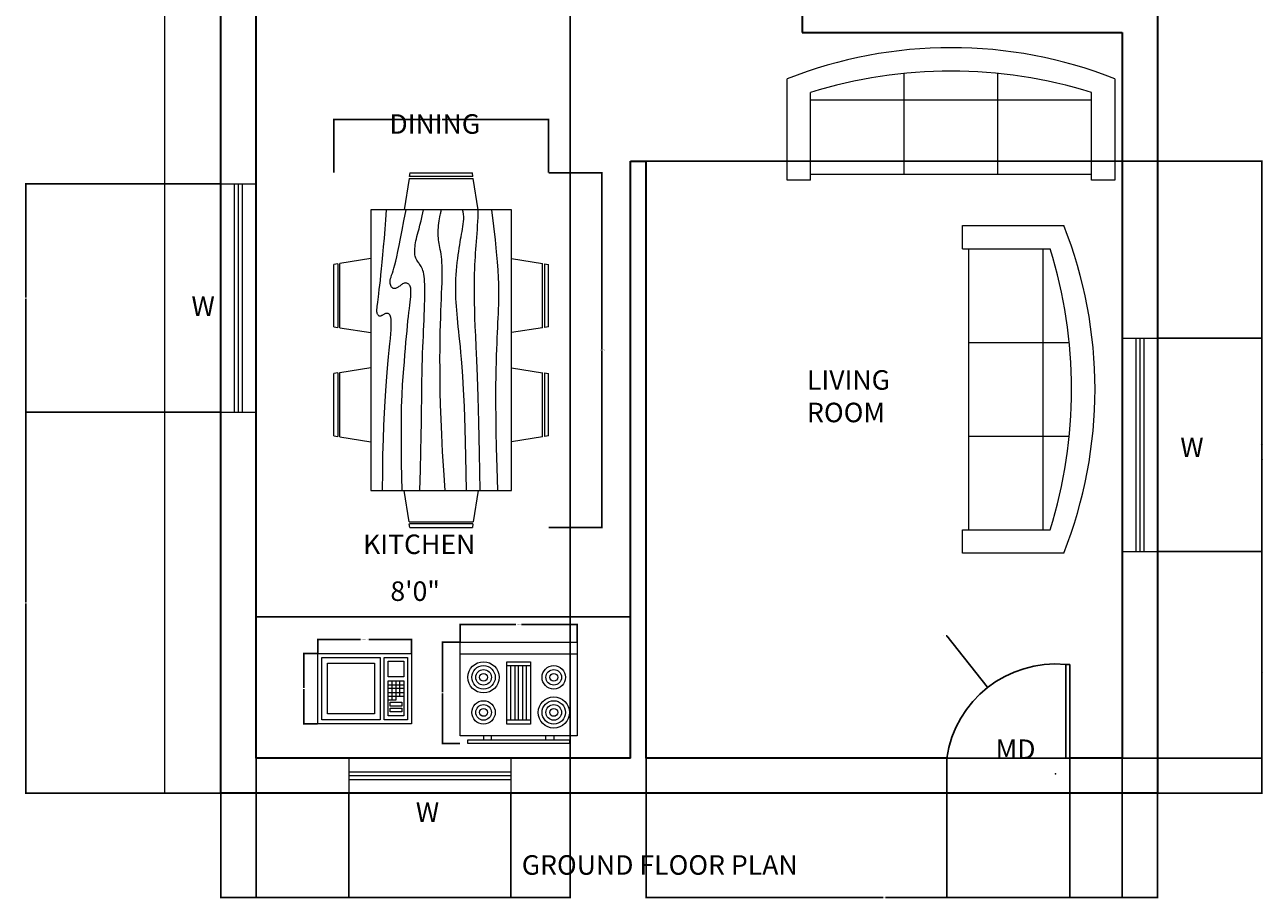
# Model space of a CAD drawing. Units: inches. Extents: x 37 to 686, y -425 to 128.
# Tile 1 of 3: x 37 to 355, y -425 to -201. Entities that reach past the tile are written whole.
import ezdxf

# ---------------------------------------------------------------- set-up
doc = ezdxf.new("R2010")
doc.units = ezdxf.units.IN
doc.header["$MEASUREMENT"] = 0
for name, color, linetype, lineweight in [('A-ANNO-DIMS', 2, 'Continuous', 13), ('A-ANNO-TEXT', 7, 'Continuous', 18), ('A-ANNO-TITL', 7, 'Continuous', 25), ('A-AREA-IDEN', 7, 'Continuous', 18), ('A-DOOR', 3, 'Continuous', 25), ('A-EQPM', 8, 'Continuous', 18), ('A-FLOR-CASE', 7, 'Continuous', 25), ('A-FURN', 8, 'Continuous', 18), ('A-GLAZ', 4, 'Continuous', 18), ('A-WALL', 7, 'Continuous', 35)]:
    doc.layers.add(name, color=color, linetype=linetype, lineweight=lineweight)
doc.styles.get("Standard").update_dxf_attribs({"font": 'arial.ttf'})
doc.dimstyles.get("Standard").update_dxf_attribs({"dimtxt": 0.18, "dimasz": 0.18, "dimexe": 0.18, "dimexo": 0.0625, "dimgap": 0.09, "dimtad": 0, "dimtih": 1, "dimtoh": 1, "dimdec": 4, "dimzin": 0, "dimdsep": 46, "dimtxsty": 'Standard', "dimcen": 0.09, "dimadec": 0, "dimazin": 0, "dimtfac": 1, "dimtdec": 4, "dimtofl": 0, "dimtmove": 0, "dimatfit": 3, "dimfxl": 1, "dimtolj": 1, "dimtzin": 0, "dimarcsym": 0})

# ---------------------------------------------------------------- blocks, each defined once
blk = doc.blocks.new('Sofa - Roundback 7 ft.')
for p, q in [((-12.00002, -32.4421), (-12.00003, -6.5971)), ((11.99997, -32.4421), (11.99998, -6.5971)), ((-36.000027, -34), (-36.000027, -11.4696)), ((35.99998, -34), (35.99998, -11.4696)), ((-35.999844, -13.3819), (35.9998, -13.3819)), ((-36.000027, -32.4421), (35.99998, -32.4421))]:
    blk.add_line(p, q)
for points in [[(-36.000027, -34), (-42.000027, -34), (-42.000027, -8)], [(41.99998, -8), (41.99998, -34), (35.99998, -34)]]:
    blk.add_lwpolyline(points)
for centre, radius, start, end in [((0, -114.25), 114.25, 68.43141, 111.5686), ((-0.00001, -127.1968), 121.1968, 72.72033, 107.2797)]:
    blk.add_arc(centre, radius, start, end)
blk = doc.blocks.new('Dining Set - 36 x 72 in.')
for p, q in [((-22.2343, 26.00059), (-23.4847, 17.99762)), ((-22.2304, 26), (-5.7608, 26)), ((-22, 27.5), (-22.1562, 26.50042)), ((-5.8416, 26.5), (-22.1534, 26.5)), ((-22, 27.5), (-6, 27.5)), ((-5.8437, 26.49966), (-6, 27.5)), ((-4.5152, 17.99762), (-5.7655, 25.99926)), ((5.7657, 26.00059), (4.5153, 17.99762)), ((5.7696, 26), (22.2392, 26)), ((6, 27.5), (5.8438, 26.50042)), ((22.1584, 26.5), (5.8466, 26.5)), ((6, 27.5), (22, 27.5)), ((22.1563, 26.49966), (22, 27.5)), ((23.4848, 17.99762), (22.2345, 25.99926)), ((36, 18), (-36, 18)), ((-36, 18), (-36, -18)), ((36, -18), (36, 18)), ((-45.5, 8), (-44.5004, 8.15617)), ((-45.5, 8), (-45.5, -8)), ((-44.5, -8.15843), (-44.5, 8.15338)), ((-44.0006, 8.23428), (-35.9976, 9.48474)), ((-44, 8.23041), (-44, -8.23915)), ((44.0006, 8.23428), (35.9976, 9.48474)), ((44, 8.23041), (44, -8.23915)), ((44.5, -8.15843), (44.5, 8.15338)), ((45.5, 8), (44.5005, 8.15617)), ((45.5, 8), (45.5, -8)), ((-44.4997, -8.15631), (-45.5, -8)), ((-35.9976, -9.48476), (-43.9993, -8.2345)), ((35.9976, -9.48476), (43.9993, -8.2345)), ((44.4997, -8.15631), (45.5, -8)), ((-36, -18), (36, -18)), ((-22.2343, -26.0006), (-23.4847, -17.99762)), ((-4.5152, -17.99762), (-5.7655, -25.99928)), ((5.7657, -26.0006), (4.5153, -17.99762)), ((23.4848, -17.99762), (22.2345, -25.99928)), ((-22.2304, -26), (-5.7608, -26)), ((-22, -27.5), (-22.1562, -26.50044)), ((-5.8416, -26.5), (-22.1534, -26.5)), ((-22, -27.5), (-6, -27.5)), ((-5.8437, -26.49967), (-6, -27.5)), ((5.7696, -26), (22.2392, -26)), ((6, -27.5), (5.8438, -26.50044)), ((22.1584, -26.5), (5.8466, -26.5)), ((6, -27.5), (22, -27.5)), ((22.1563, -26.49967), (22, -27.5))]:
    blk.add_line(p, q)
for points in [[(-36, 15), (-31.1772, 14.97754), (-26.8079, 14.91406), (-22.8538, 14.81543), (-19.276, 14.6875), (-16.0362, 14.53613), (-13.0957, 14.36718), (-10.4159, 14.18652), (-7.9583, 14), (-5.6904, 13.81315), (-3.6035, 13.63021), (-1.6954, 13.45508), (0.0365, 13.29166), (1.5945, 13.14388), (2.9811, 13.01562), (4.1988, 12.9108), (5.25, 12.83333), (6.1393, 12.78613), (6.8802, 12.76823), (7.4883, 12.77767), (7.9792, 12.8125), (8.3685, 12.87077), (8.6719, 12.95052), (8.9049, 13.0498), (9.0833, 13.16666), (9.2205, 13.29899), (9.3216, 13.44401), (9.3895, 13.59879), (9.4271, 13.76041), (9.4373, 13.92594), (9.4232, 14.09245), (9.3875, 14.257), (9.3333, 14.41666), (9.2638, 14.56917), (9.1836, 14.71484), (9.0975, 14.85465), (9.0104, 14.98958), (8.9272, 15.1206), (8.8529, 15.2487), (8.7922, 15.37483), (8.75, 15.5), (8.7305, 15.62467), (8.7344, 15.74739), (8.7617, 15.86621), (8.8125, 15.97916), (8.8867, 16.08431), (8.9844, 16.17968), (9.1055, 16.26334), (9.25, 16.33333), (9.4189, 16.38802), (9.6172, 16.42708), (9.8506, 16.45052), (10.125, 16.45833), (10.4463, 16.45052), (10.8203, 16.42708), (11.2529, 16.38802), (11.75, 16.33333), (12.3184, 16.26318), (12.9694, 16.17838), (13.7151, 16.07991), (14.5677, 15.96875), (15.5395, 15.84586), (16.6426, 15.71224), (17.8893, 15.56884), (19.2917, 15.41666), (20.859, 15.25667), (22.5879, 15.08984), (24.4721, 14.91715), (26.5052, 14.73958), (28.6809, 14.5581), (30.9929, 14.3737), (33.4347, 14.18733), (36, 14)], [(-36, 10), (-28.9766, 10.14274), (-23.1725, 10.20442), (-18.4241, 10.19775), (-14.5677, 10.13541), (-11.4399, 10.03011), (-8.877, 9.89453), (-6.7154, 9.74137), (-4.7917, 9.58333), (-2.9698, 9.43082), (-1.2246, 9.28515), (0.4415, 9.14534), (2.026, 9.01041), (3.5266, 8.87939), (4.9408, 8.7513), (6.266, 8.62516), (7.5, 8.5), (8.6411, 8.37549), (9.6914, 8.2539), (10.6538, 8.13818), (11.5312, 8.03125), (12.3267, 7.93603), (13.043, 7.85547), (13.6831, 7.79248), (14.25, 7.75), (14.7471, 7.7303), (15.1797, 7.73307), (15.5537, 7.75732), (15.875, 7.80208), (16.1494, 7.86637), (16.3828, 7.94922), (16.5811, 8.04964), (16.75, 8.16666), (16.8944, 8.29915), (17.0143, 8.44531), (17.1089, 8.60319), (17.1771, 8.77083), (17.218, 8.94629), (17.2305, 9.1276), (17.2137, 9.31282), (17.1667, 9.5), (17.0895, 9.6875), (16.987, 9.875), (16.8649, 10.0625), (16.7292, 10.25), (16.5856, 10.4375), (16.4401, 10.625), (16.2985, 10.8125), (16.1667, 11), (16.05, 11.18733), (15.9518, 11.3737), (15.8752, 11.5581), (15.8229, 11.73958), (15.798, 11.91715), (15.8034, 12.08984), (15.842, 12.25667), (15.9167, 12.41666), (16.0295, 12.56836), (16.1784, 12.70833), (16.3605, 12.83268), (16.5729, 12.9375), (16.8127, 13.01888), (17.0768, 13.07291), (17.3625, 13.0957), (17.6667, 13.08333), (17.9894, 13.03312), (18.3418, 12.94726), (18.7382, 12.82918), (19.1927, 12.68229), (19.7195, 12.51001), (20.3327, 12.31575), (21.0465, 12.10294), (21.875, 11.875), (22.8357, 11.63354), (23.959, 11.37304), (25.2786, 11.08618), (26.8282, 10.76562), (28.6414, 10.40405), (30.752, 9.99414), (33.1936, 9.52856), (36, 9)], [(-36, 5.5), (-30.7157, 5.3348), (-26.069, 5.20963), (-21.9946, 5.11767), (-18.4271, 5.05208), (-15.3009, 5.00602), (-12.5508, 4.97265), (-10.1112, 4.94515), (-7.9167, 4.91666), (-5.909, 4.88167), (-4.0586, 4.83984), (-2.3429, 4.79215), (-0.7396, 4.73958), (0.7739, 4.6831), (2.22, 4.6237), (3.6213, 4.56233), (5, 4.5), (6.373, 4.43782), (7.7344, 4.3776), (9.0723, 4.32129), (10.375, 4.27083), (11.6309, 4.22819), (12.8281, 4.19531), (13.9551, 4.17415), (15, 4.16666), (15.954, 4.17448), (16.819, 4.19791), (17.6001, 4.23698), (18.3021, 4.29166), (18.9299, 4.36198), (19.4883, 4.44791), (19.9823, 4.54948), (20.4167, 4.66666), (20.7969, 4.79899), (21.1302, 4.94401), (21.4245, 5.09879), (21.6875, 5.26041), (21.9271, 5.42594), (22.1511, 5.59245), (22.3672, 5.757), (22.5834, 5.91666), (22.8065, 6.06868), (23.0404, 6.21093), (23.2879, 6.34147), (23.5521, 6.45833), (23.8358, 6.55957), (24.142, 6.64323), (24.4735, 6.70735), (24.8334, 6.75), (25.2235, 6.76969), (25.642, 6.76692), (26.0858, 6.74267), (26.5521, 6.69791), (27.0379, 6.63362), (27.5404, 6.55078), (28.0565, 6.45036), (28.5834, 6.33333), (29.1242, 6.19987), (29.7071, 6.04687), (30.3661, 5.87044), (31.1354, 5.66666), (32.0493, 5.43164), (33.142, 5.16146), (34.4475, 4.85221), (36, 4.5)], [(-36, -1), (-30.7915, -0.6591), (-26.0195, -0.38216), (-21.6519, -0.16284), (-17.6563, 0.00521), (-14.0005, 0.12833), (-10.6523, 0.21289), (-7.5796, 0.26522), (-4.75, 0.29166), (-2.134, 0.29793), (0.2878, 0.28711), (2.5317, 0.26163), (4.6146, 0.22396), (6.5529, 0.17651), (8.3633, 0.12174), (10.0623, 0.06209), (11.6667, 0), (13.1899, -0.06201), (14.6341, -0.1211), (15.9982, -0.17432), (17.2813, -0.21875), (18.4823, -0.25147), (19.6003, -0.26953), (20.6343, -0.27002), (21.5834, -0.25), (22.4481, -0.20768), (23.2357, -0.14584), (23.9549, -0.06836), (24.6146, 0.02083), (25.2235, 0.11784), (25.7904, 0.21875), (26.3241, 0.31966), (26.8334, 0.41666), (27.3265, 0.50618), (27.8099, 0.58593), (28.2894, 0.65397), (28.7709, 0.70833), (29.2601, 0.74707), (29.763, 0.76823), (30.2855, 0.76985), (30.8334, 0.75), (31.4088, 0.70784), (31.9994, 0.64713), (32.589, 0.57275), (33.1615, 0.48958), (33.7008, 0.4025), (34.1908, 0.3164), (34.6153, 0.23616), (34.9584, 0.16666), (35.2099, 0.11165), (35.3848, 0.07031), (35.504, 0.04069), (35.5886, 0.02083), (35.6594, 0.00879), (35.7377, 0.0026), (35.8442, 0.00032), (36, 0)], [(-36, -6.5), (-27.1843, -6.31267), (-20.084, -6.1263), (-14.469, -5.9419), (-10.1094, -5.76042), (-6.7752, -5.58285), (-4.2363, -5.41016), (-2.2629, -5.24333), (-0.625, -5.08334), (0.8708, -4.93099), (2.2715, -4.78646), (3.5872, -4.64974), (4.8281, -4.52084), (6.0046, -4.39974), (7.127, -4.28646), (8.2053, -4.18099), (9.25, -4.08334), (10.2705, -3.99382), (11.2734, -3.91407), (12.2647, -3.84603), (13.25, -3.79167), (14.2354, -3.75293), (15.2266, -3.73177), (16.2295, -3.73015), (17.25, -3.75), (18.2912, -3.79248), (19.3451, -3.85547), (20.4009, -3.93604), (21.4479, -4.03125), (22.4754, -4.13819), (23.4727, -4.25391), (24.4289, -4.37549), (25.3334, -4.5), (26.1785, -4.62492), (26.9694, -4.74935), (27.7145, -4.87281), (28.4219, -4.99479), (29.1, -5.11483), (29.7572, -5.23242), (30.4016, -5.34709), (31.0417, -5.45834), (31.6837, -5.56437), (32.3262, -5.65821), (32.9658, -5.73153), (33.599, -5.77604), (34.2224, -5.78345), (34.8327, -5.74545), (35.4264, -5.65373), (36, -5.5)], [(-36, -10), (-26.4022, -9.81299), (-18.4675, -9.62891), (-11.9839, -9.45069), (-6.7396, -9.28125), (-2.5226, -9.12354), (0.8789, -8.98047), (3.6769, -8.85498), (6.0833, -8.75), (8.2767, -8.66765), (10.3021, -8.60677), (12.1712, -8.56543), (13.8958, -8.54167), (15.4876, -8.53353), (16.9583, -8.53907), (18.3197, -8.55632), (19.5834, -8.58334), (20.7616, -8.61841), (21.8685, -8.66081), (22.9188, -8.71004), (23.9271, -8.76563), (24.9081, -8.82707), (25.8763, -8.89388), (26.8465, -8.96558), (27.8334, -9.04167), (28.8474, -9.12118), (29.8828, -9.20117), (30.93, -9.27824), (31.9792, -9.34896), (33.0205, -9.40991), (34.0443, -9.45768), (35.0407, -9.48885), (36, -9.5)], [(-36, -14.5), (-30.0881, -14.33513), (-25.0332, -14.21224), (-20.7312, -14.12647), (-17.0781, -14.07292), (-13.97, -14.04671), (-11.3027, -14.04297), (-8.9724, -14.05681), (-6.875, -14.08334), (-4.9224, -14.11833), (-3.0905, -14.16016), (-1.3709, -14.20785), (0.2448, -14.26042), (1.7647, -14.3169), (3.1973, -14.3763), (4.5507, -14.43767), (5.8333, -14.5), (7.0554, -14.5621), (8.235, -14.62175), (9.3922, -14.67652), (10.5469, -14.72396), (11.7192, -14.76164), (12.929, -14.78711), (14.1965, -14.79794), (15.5417, -14.79167), (16.9933, -14.76424), (18.6152, -14.70508), (20.4804, -14.60197), (22.6615, -14.44271), (25.2312, -14.21509), (28.2624, -13.9069), (31.8277, -13.50594), (36, -13)]]:
    blk.add_lwpolyline(points)
blk = doc.blocks.new('Range-Oven - 30 in top')
for p, q in [((0, -3), (30, -3)), ((12, -6), (18, -6)), ((13, -20), (13, -6)), ((14, -6), (14, -20)), ((15, -20), (15, -6)), ((16, -6), (16, -20)), ((17, -20), (17, -6)), ((18, -20), (12, -20)), ((6, -24), (6, -25)), ((8, -25), (8, -24)), ((22, -25), (22, -24)), ((24, -24), (24, -25))]:
    blk.add_line(p, q)
for points in [[(0, -24), (0, 0), (30, 0), (30, -24)], [(12, -21), (12, -5), (18, -5), (18, -21)], [(2, -26), (2, -25), (28, -25), (28, -26)]]:
    blk.add_lwpolyline(points, close=True)
for centre, radius in [((6, -9), 4), ((6, -9), 3), ((24, -9), 3), ((6, -9), 2), ((6, -9), 1), ((24, -9), 2), ((24, -9), 1), ((6, -18), 3), ((24, -18), 4), ((24, -18), 3), ((6, -18), 2), ((6, -18), 1), ((24, -18), 2), ((24, -18), 1)]:
    blk.add_circle(centre, radius)
blk = doc.blocks.new('Microwave')
for p, q in [((18, 10), (22, 10)), ((19, 7), (19, 11)), ((20, 11), (20, 7)), ((21, 7), (21, 11)), ((22, 9), (18, 9)), ((18, 8), (22, 8)), ((22, 7), (18, 7)), ((19, 6), (19, 7)), ((20, 7), (20, 6)), ((20, 6), (18, 6))]:
    blk.add_line(p, q)
for points in [[(0, 0), (0, 18), (24, 18), (24, 0)], [(1, 1), (1, 17), (16, 17), (16, 1)], [(17, 1), (17, 17), (23, 17), (23, 1)], [(18, 12), (18, 16), (22, 16), (22, 12)], [(2.5, 2.5), (2.5, 15.5), (14.5, 15.5), (14.5, 2.5)], [(18, 2), (18, 11), (22, 11), (22, 2)], [(18.5, 4.5), (18.5, 5.5), (21.5, 5.5), (21.5, 4.5)], [(18.5, 3), (18.5, 4), (21.5, 4), (21.5, 3)]]:
    blk.add_lwpolyline(points, close=True)
blk = doc.blocks.new('DOOR-LEAF-24IN')
for p, q in [((0, 0), (0, 24)), ((0, 24), (1, 24)), ((1, 24), (1, 0)), ((1, 0), (0, 0))]:
    blk.add_line(p, q)
blk = doc.blocks.new('*D16')
at = {"layer": 'A-ANNO-DIMS', "color": 0, "lineweight": -2, "transparency": 16777216}
for p, q in [((171.63, -239.15), (185.4, -239.15)), ((185.22, -239.33), (185.22, -284.47)), ((185.22, -329.97), (185.22, -284.84)), ((171.63, -330.15), (185.4, -330.15))]:
    blk.add_line(p, q, dxfattribs=at)
at = {"layer": 'A-ANNO-DIMS', "color": 0, "transparency": 16777216}
for points in [[(185.19, -239.33), (185.25, -239.33), (185.22, -239.15)], [(185.19, -329.97), (185.25, -329.97), (185.22, -330.15)]]:
    blk.add_solid(points, dxfattribs=at)
at = {"layer": 'Defpoints', "color": 0, "transparency": 16777216}
for p in [(171.57, -239.15), (185.22, -239.15), (171.57, -330.15)]:
    blk.add_point(p, dxfattribs=at)
at = {"layer": 'A-ANNO-DIMS', "color": 0, "transparency": 16777216, "insert": (185.22, -284.65), "char_height": 0.18, "attachment_point": 5}
blk.add_mtext('\\A1;DINING SET 91', dxfattribs=at)
blk = doc.blocks.new('*D17')
at = {"layer": 'A-ANNO-DIMS', "color": 0, "lineweight": -2, "transparency": 16777216}
for p, q in [((116.57, -239.09), (116.57, -225.32)), ((171.57, -239.09), (171.57, -225.32)), ((116.75, -225.5), (143.85, -225.5)), ((171.39, -225.5), (144.29, -225.5))]:
    blk.add_line(p, q, dxfattribs=at)
at = {"layer": 'A-ANNO-DIMS', "color": 0, "transparency": 16777216}
for points in [[(116.75, -225.47), (116.75, -225.53), (116.57, -225.5)], [(171.39, -225.47), (171.39, -225.53), (171.57, -225.5)]]:
    blk.add_solid(points, dxfattribs=at)
at = {"layer": 'Defpoints', "color": 0, "transparency": 16777216}
for p in [(116.57, -225.5), (116.57, -239.15), (171.57, -239.15)]:
    blk.add_point(p, dxfattribs=at)
at = {"layer": 'A-ANNO-DIMS', "color": 0, "transparency": 16777216, "insert": (144.07, -225.5), "char_height": 0.18, "attachment_point": 5}
blk.add_mtext('\\A1;55', dxfattribs=at)
blk = doc.blocks.new('*D18')
at = {"layer": 'A-ANNO-DIMS', "color": 0, "lineweight": -2, "transparency": 16777216}
for p, q in [((148.93, -359.46), (148.93, -354.84)), ((149.11, -355.02), (163.24, -355.02)), ((178.75, -355.02), (164.63, -355.02)), ((178.93, -359.46), (178.93, -354.84))]:
    blk.add_line(p, q, dxfattribs=at)
at = {"layer": 'A-ANNO-DIMS', "color": 0, "transparency": 16777216}
for points in [[(149.11, -354.99), (149.11, -355.05), (148.93, -355.02)], [(178.75, -354.99), (178.75, -355.05), (178.93, -355.02)]]:
    blk.add_solid(points, dxfattribs=at)
at = {"layer": 'Defpoints', "color": 0, "transparency": 16777216}
for p in [(178.93, -355.02), (148.93, -359.52), (178.93, -359.52)]:
    blk.add_point(p, dxfattribs=at)
at = {"layer": 'A-ANNO-DIMS', "color": 0, "transparency": 16777216, "insert": (163.93, -355.02), "char_height": 0.18, "attachment_point": 5}
blk.add_mtext('\\A1;RANGE 30', dxfattribs=at)
blk = doc.blocks.new('*D19')
at = {"layer": 'A-ANNO-DIMS', "color": 0, "lineweight": -2, "transparency": 16777216}
for p, q in [((148.87, -359.52), (144.25, -359.52)), ((144.43, -359.7), (144.43, -372.34)), ((144.43, -385.34), (144.43, -372.7)), ((148.87, -385.52), (144.25, -385.52))]:
    blk.add_line(p, q, dxfattribs=at)
at = {"layer": 'A-ANNO-DIMS', "color": 0, "transparency": 16777216}
for points in [[(144.4, -359.7), (144.46, -359.7), (144.43, -359.52)], [(144.4, -385.34), (144.46, -385.34), (144.43, -385.52)]]:
    blk.add_solid(points, dxfattribs=at)
at = {"layer": 'Defpoints', "color": 0, "transparency": 16777216}
for p in [(144.43, -359.52), (148.93, -359.52), (148.93, -385.52)]:
    blk.add_point(p, dxfattribs=at)
at = {"layer": 'A-ANNO-DIMS', "color": 0, "transparency": 16777216, "insert": (144.43, -372.52), "char_height": 0.18, "attachment_point": 5}
blk.add_mtext('\\A1;26', dxfattribs=at)
blk = doc.blocks.new('*D20')
at = {"layer": 'A-ANNO-DIMS', "color": 0, "lineweight": -2, "transparency": 16777216}
for p, q in [((112.48, -362.35), (112.48, -358.63)), ((136.48, -362.35), (136.48, -358.63)), ((112.66, -358.81), (123.44, -358.81)), ((136.3, -358.81), (125.52, -358.81))]:
    blk.add_line(p, q, dxfattribs=at)
at = {"layer": 'A-ANNO-DIMS', "color": 0, "transparency": 16777216}
for points in [[(112.66, -358.78), (112.66, -358.84), (112.48, -358.81)], [(136.3, -358.78), (136.3, -358.84), (136.48, -358.81)]]:
    blk.add_solid(points, dxfattribs=at)
at = {"layer": 'Defpoints', "color": 0, "transparency": 16777216}
for p in [(136.48, -358.81), (112.48, -362.41), (136.48, -362.41)]:
    blk.add_point(p, dxfattribs=at)
at = {"layer": 'A-ANNO-DIMS', "color": 0, "transparency": 16777216, "insert": (124.48, -358.81), "char_height": 0.18, "attachment_point": 5}
blk.add_mtext('\\A1;MICROWAVE 24', dxfattribs=at)
blk = doc.blocks.new('*D21')
at = {"layer": 'A-ANNO-DIMS', "color": 0, "lineweight": -2, "transparency": 16777216}
for p, q in [((112.42, -362.41), (108.7, -362.41)), ((108.88, -362.59), (108.88, -371.23)), ((108.88, -380.23), (108.88, -371.59)), ((112.42, -380.41), (108.7, -380.41))]:
    blk.add_line(p, q, dxfattribs=at)
at = {"layer": 'A-ANNO-DIMS', "color": 0, "transparency": 16777216}
for points in [[(108.85, -362.59), (108.91, -362.59), (108.88, -362.41)], [(108.85, -380.23), (108.91, -380.23), (108.88, -380.41)]]:
    blk.add_solid(points, dxfattribs=at)
at = {"layer": 'Defpoints', "color": 0, "transparency": 16777216}
for p in [(108.88, -362.41), (112.48, -362.41), (112.48, -380.41)]:
    blk.add_point(p, dxfattribs=at)
at = {"layer": 'A-ANNO-DIMS', "color": 0, "transparency": 16777216, "insert": (108.88, -371.41), "char_height": 0.18, "attachment_point": 5}
blk.add_mtext('\\A1;18', dxfattribs=at)
blk = doc.blocks.new('*D23')
at = {"layer": 'A-ANNO-DIMS', "color": 0, "lineweight": -2, "transparency": 16777216}
for p, q in [((96.63, -51.29), (96.63, -425.16)), ((177.14, -51.29), (177.14, -425.16)), ((96.81, -424.98), (136.56, -424.98)), ((176.96, -424.98), (137.21, -424.98))]:
    blk.add_line(p, q, dxfattribs=at)
at = {"layer": 'A-ANNO-DIMS', "color": 0, "transparency": 16777216}
for points in [[(96.81, -424.95), (96.81, -425.01), (96.63, -424.98)], [(176.96, -424.95), (176.96, -425.01), (177.14, -424.98)]]:
    blk.add_solid(points, dxfattribs=at)
at = {"layer": 'Defpoints', "color": 0, "transparency": 16777216}
for p in [(96.63, -51.23), (177.14, -51.23), (177.14, -424.98)]:
    blk.add_point(p, dxfattribs=at)
at = {"layer": 'A-ANNO-DIMS', "color": 0, "transparency": 16777216, "insert": (136.88, -424.98), "char_height": 0.18, "attachment_point": 5}
blk.add_mtext('\\A1;80.5', dxfattribs=at)
blk = doc.blocks.new('*D24')
at = {"layer": 'A-ANNO-DIMS', "color": 0, "lineweight": -2, "transparency": 16777216}
for p, q in [((196.63, -389.29), (196.63, -425.16)), ((318.63, -389.29), (318.63, -425.16)), ((196.81, -424.98), (257.35, -424.98)), ((318.45, -424.98), (257.91, -424.98))]:
    blk.add_line(p, q, dxfattribs=at)
at = {"layer": 'A-ANNO-DIMS', "color": 0, "transparency": 16777216}
for points in [[(196.81, -424.95), (196.81, -425.01), (196.63, -424.98)], [(318.45, -424.95), (318.45, -425.01), (318.63, -424.98)]]:
    blk.add_solid(points, dxfattribs=at)
at = {"layer": 'Defpoints', "color": 0, "transparency": 16777216}
for p in [(196.63, -389.23), (318.63, -389.23), (196.63, -424.98)]:
    blk.add_point(p, dxfattribs=at)
at = {"layer": 'A-ANNO-DIMS', "color": 0, "transparency": 16777216, "insert": (257.63, -424.98), "char_height": 0.18, "attachment_point": 5}
blk.add_mtext('\\A1;122', dxfattribs=at)
blk = doc.blocks.new('*D25')
at = {"layer": 'A-ANNO-DIMS', "color": 0, "lineweight": -2, "transparency": 16777216}
for p, q in [((196.69, -236.17), (354.56, -236.17)), ((354.38, -236.35), (354.38, -312.51)), ((354.38, -389.05), (354.38, -312.88)), ((196.69, -389.23), (354.56, -389.23))]:
    blk.add_line(p, q, dxfattribs=at)
at = {"layer": 'A-ANNO-DIMS', "color": 0, "transparency": 16777216}
for points in [[(354.35, -236.35), (354.41, -236.35), (354.38, -236.17)], [(354.35, -389.05), (354.41, -389.05), (354.38, -389.23)]]:
    blk.add_solid(points, dxfattribs=at)
at = {"layer": 'Defpoints', "color": 0, "transparency": 16777216}
for p in [(196.63, -236.17), (196.63, -389.23), (354.38, -389.23)]:
    blk.add_point(p, dxfattribs=at)
at = {"layer": 'A-ANNO-DIMS', "color": 0, "transparency": 16777216, "insert": (354.38, -312.7), "char_height": 0.18, "attachment_point": 5}
blk.add_mtext('\\A1;153.06', dxfattribs=at)
blk = doc.blocks.new('*D31')
at = {"layer": 'A-ANNO-DIMS', "color": 0, "lineweight": -2, "transparency": 16777216}
for p, q in [((87.57, -242.02), (37.48, -242.02)), ((37.66, -242.2), (37.66, -271.12)), ((37.66, -300.39), (37.66, -271.48)), ((87.57, -300.57), (37.48, -300.57))]:
    blk.add_line(p, q, dxfattribs=at)
at = {"layer": 'A-ANNO-DIMS', "color": 0, "transparency": 16777216}
for points in [[(37.63, -242.2), (37.69, -242.2), (37.66, -242.02)], [(37.63, -300.39), (37.69, -300.39), (37.66, -300.57)]]:
    blk.add_solid(points, dxfattribs=at)
at = {"layer": 'Defpoints', "color": 0, "transparency": 16777216}
for p in [(37.66, -242.02), (87.63, -242.02), (87.63, -300.57)]:
    blk.add_point(p, dxfattribs=at)
at = {"layer": 'A-ANNO-DIMS', "color": 0, "transparency": 16777216, "insert": (37.66, -271.3), "char_height": 0.18, "attachment_point": 5}
blk.add_mtext('\\A1;58.55', dxfattribs=at)
blk = doc.blocks.new('*D32')
at = {"layer": 'A-ANNO-DIMS', "color": 0, "lineweight": -2, "transparency": 16777216}
for p, q in [((327.69, -281.56), (354.56, -281.56)), ((354.38, -281.74), (354.38, -308.73)), ((354.38, -336.08), (354.38, -309.09)), ((327.69, -336.26), (354.56, -336.26))]:
    blk.add_line(p, q, dxfattribs=at)
at = {"layer": 'A-ANNO-DIMS', "color": 0, "transparency": 16777216}
for points in [[(354.35, -281.74), (354.41, -281.74), (354.38, -281.56)], [(354.35, -336.08), (354.41, -336.08), (354.38, -336.26)]]:
    blk.add_solid(points, dxfattribs=at)
at = {"layer": 'Defpoints', "color": 0, "transparency": 16777216}
for p in [(327.63, -281.56), (354.38, -281.56), (327.63, -336.26)]:
    blk.add_point(p, dxfattribs=at)
at = {"layer": 'A-ANNO-DIMS', "color": 0, "transparency": 16777216, "insert": (354.38, -308.91), "char_height": 0.18, "attachment_point": 5}
blk.add_mtext('\\A1;54.69', dxfattribs=at)
blk = doc.blocks.new('*D35')
at = {"layer": 'A-ANNO-DIMS', "color": 0, "lineweight": -2, "transparency": 16777216}
for p, q in [((120.41, -398.29), (120.41, -425.16)), ((161.96, -398.29), (161.96, -425.16)), ((120.59, -424.98), (140.79, -424.98)), ((161.78, -424.98), (141.58, -424.98))]:
    blk.add_line(p, q, dxfattribs=at)
at = {"layer": 'A-ANNO-DIMS', "color": 0, "transparency": 16777216}
for points in [[(120.59, -424.95), (120.59, -425.01), (120.41, -424.98)], [(161.78, -424.95), (161.78, -425.01), (161.96, -424.98)]]:
    blk.add_solid(points, dxfattribs=at)
at = {"layer": 'Defpoints', "color": 0, "transparency": 16777216}
for p in [(120.41, -398.23), (161.96, -398.23), (161.96, -424.98)]:
    blk.add_point(p, dxfattribs=at)
at = {"layer": 'A-ANNO-DIMS', "color": 0, "transparency": 16777216, "insert": (141.18, -424.98), "char_height": 0.18, "attachment_point": 5}
blk.add_mtext('\\A1;41.54', dxfattribs=at)
blk = doc.blocks.new('*D43')
at = {"layer": 'A-ANNO-DIMS', "color": 0, "lineweight": -2, "transparency": 16777216}
for p, q in [((87.57, -300.57), (37.48, -300.57)), ((37.66, -300.75), (37.66, -349.22)), ((37.66, -398.05), (37.66, -349.58)), ((87.57, -398.23), (37.48, -398.23))]:
    blk.add_line(p, q, dxfattribs=at)
at = {"layer": 'A-ANNO-DIMS', "color": 0, "transparency": 16777216}
for points in [[(37.63, -300.75), (37.69, -300.75), (37.66, -300.57)], [(37.63, -398.05), (37.69, -398.05), (37.66, -398.23)]]:
    blk.add_solid(points, dxfattribs=at)
at = {"layer": 'Defpoints', "color": 0, "transparency": 16777216}
for p in [(37.66, -300.57), (87.63, -300.57), (87.63, -398.23)]:
    blk.add_point(p, dxfattribs=at)
at = {"layer": 'A-ANNO-DIMS', "color": 0, "transparency": 16777216, "insert": (37.66, -349.4), "char_height": 0.18, "attachment_point": 5}
blk.add_mtext('\\A1;97.65', dxfattribs=at)
blk = doc.blocks.new('*D44')
at = {"layer": 'A-ANNO-DIMS', "color": 0, "lineweight": -2, "transparency": 16777216}
for p, q in [((327.69, -336.26), (354.56, -336.26)), ((354.38, -336.44), (354.38, -367.06)), ((354.38, -398.05), (354.38, -367.42)), ((327.69, -398.23), (354.56, -398.23))]:
    blk.add_line(p, q, dxfattribs=at)
at = {"layer": 'A-ANNO-DIMS', "color": 0, "transparency": 16777216}
for points in [[(354.35, -336.44), (354.41, -336.44), (354.38, -336.26)], [(354.35, -398.05), (354.41, -398.05), (354.38, -398.23)]]:
    blk.add_solid(points, dxfattribs=at)
at = {"layer": 'Defpoints', "color": 0, "transparency": 16777216}
for p in [(327.63, -336.26), (354.38, -336.26), (327.63, -398.23)]:
    blk.add_point(p, dxfattribs=at)
at = {"layer": 'A-ANNO-DIMS', "color": 0, "transparency": 16777216, "insert": (354.38, -367.24), "char_height": 0.18, "attachment_point": 5}
blk.add_mtext('\\A1;61.97', dxfattribs=at)
blk = doc.blocks.new('*D47')
at = {"layer": 'A-ANNO-DIMS', "color": 0, "lineweight": -2, "transparency": 16777216}
for p, q in [((87.63, -398.29), (87.63, -425.16)), ((120.41, -398.29), (120.41, -425.16)), ((87.81, -424.98), (103.63, -424.98)), ((120.23, -424.98), (104.42, -424.98))]:
    blk.add_line(p, q, dxfattribs=at)
at = {"layer": 'A-ANNO-DIMS', "color": 0, "transparency": 16777216}
for points in [[(87.81, -424.95), (87.81, -425.01), (87.63, -424.98)], [(120.23, -424.95), (120.23, -425.01), (120.41, -424.98)]]:
    blk.add_solid(points, dxfattribs=at)
at = {"layer": 'Defpoints', "color": 0, "transparency": 16777216}
for p in [(87.63, -398.23), (120.41, -398.23), (120.41, -424.98)]:
    blk.add_point(p, dxfattribs=at)
at = {"layer": 'A-ANNO-DIMS', "color": 0, "transparency": 16777216, "insert": (104.02, -424.98), "char_height": 0.18, "attachment_point": 5}
blk.add_mtext('\\A1;32.78', dxfattribs=at)
blk = doc.blocks.new('*D53')
at = {"layer": 'A-ANNO-DIMS', "color": 0, "lineweight": -2, "transparency": 16777216}
for p, q in [((273.67, -398.29), (273.67, -425.16)), ((305.16, -398.29), (305.16, -425.16)), ((273.85, -424.98), (288.95, -424.98)), ((304.98, -424.98), (289.88, -424.98))]:
    blk.add_line(p, q, dxfattribs=at)
at = {"layer": 'A-ANNO-DIMS', "color": 0, "transparency": 16777216}
for points in [[(273.85, -424.95), (273.85, -425.01), (273.67, -424.98)], [(304.98, -424.95), (304.98, -425.01), (305.16, -424.98)]]:
    blk.add_solid(points, dxfattribs=at)
at = {"layer": 'Defpoints', "color": 0, "transparency": 16777216}
for p in [(273.67, -398.23), (305.16, -398.23), (305.16, -424.98)]:
    blk.add_point(p, dxfattribs=at)
at = {"layer": 'A-ANNO-DIMS', "color": 0, "transparency": 16777216, "insert": (289.41, -424.98), "char_height": 0.18, "attachment_point": 5}
blk.add_mtext('\\A1;31.484', dxfattribs=at)
blk = doc.blocks.new('*D54')
at = {"layer": 'A-ANNO-DIMS', "color": 0, "lineweight": -2, "transparency": 16777216}
for p, q in [((305.16, -398.29), (305.16, -425.16)), ((327.63, -398.29), (327.63, -425.16)), ((305.34, -424.98), (315.93, -424.98)), ((327.45, -424.98), (316.86, -424.98))]:
    blk.add_line(p, q, dxfattribs=at)
at = {"layer": 'A-ANNO-DIMS', "color": 0, "transparency": 16777216}
for points in [[(305.34, -424.95), (305.34, -425.01), (305.16, -424.98)], [(327.45, -424.95), (327.45, -425.01), (327.63, -424.98)]]:
    blk.add_solid(points, dxfattribs=at)
at = {"layer": 'Defpoints', "color": 0, "transparency": 16777216}
for p in [(305.16, -398.23), (327.63, -398.23), (327.63, -424.98)]:
    blk.add_point(p, dxfattribs=at)
at = {"layer": 'A-ANNO-DIMS', "color": 0, "transparency": 16777216, "insert": (316.39, -424.98), "char_height": 0.18, "attachment_point": 5}
blk.add_mtext('\\A1;22.476', dxfattribs=at)
blk = doc.blocks.new('*D66')
at = {"layer": 'A-ANNO-DIMS', "color": 0, "lineweight": -2, "transparency": 16777216}
for p, q in [((273.49, -357.86), (273.67, -357.86)), ((273.67, -357.86), (284.01, -371)), ((301.45, -393.27), (301.63, -393.27)), ((301.54, -393.36), (301.54, -393.18))]:
    blk.add_line(p, q, dxfattribs=at)
at = {"layer": 'A-ANNO-DIMS', "color": 0, "transparency": 16777216}
blk.add_solid([(284.03, -370.98), (283.99, -371.02), (284.12, -371.14)], dxfattribs=at)
at = {"layer": 'Defpoints', "color": 0, "transparency": 16777216}
for p in [(284.12, -371.14), (301.54, -393.27)]:
    blk.add_point(p, dxfattribs=at)
at = {"layer": 'A-ANNO-DIMS', "color": 0, "transparency": 16777216, "insert": (273.01, -357.86), "char_height": 0.18, "attachment_point": 5}
blk.add_mtext('\\A1;R28.16', dxfattribs=at)

msp = doc.modelspace()

# ---------------------------------------------------------------- linework, layer by layer
at = {"layer": 'A-ANNO-DIMS'}
for p, q in [((73.1317, -145.9359), (73.1317, -398.2271)), ((73.9598, -398.2271), (67.1024, -398.2271)), ((83.6199, -398.2271), (73.9598, -398.2271))]:
    msp.add_line(p, q, dxfattribs=at)
at = {"layer": 'A-DOOR'}
for p, q in [((273.6719, -389.2271), (273.6719, -398.2271)), ((305.1559, -389.2271), (305.1559, -398.2271))]:
    msp.add_line(p, q, dxfattribs=at)
msp.add_arc((301.5424, -393.2675), 28.1619, 84.675213, 171.751363, dxfattribs=at)
at = {"layer": 'A-FLOR-CASE'}
msp.add_line((192.6318, -353.0276), (96.6318, -353.0276), dxfattribs=at)
at = {"layer": 'A-GLAZ'}
for p, q in [((87.6318, -242.023), (96.6318, -242.023)), ((91.1318, -300.5736), (91.1318, -242.023)), ((91.1318, -300.5736), (91.1318, -242.023)), ((92.1318, -300.5736), (92.1318, -242.023)), ((93.1318, -300.5736), (93.1318, -242.023)), ((318.6318, -281.5645), (327.6318, -281.5645)), ((322.1318, -281.5645), (322.1318, -336.2564)), ((323.1318, -281.5645), (323.1318, -336.2564)), ((324.1318, -281.5645), (324.1318, -336.2564)), ((87.6318, -300.5736), (96.6318, -300.5736)), ((318.6318, -336.2564), (327.6318, -336.2564)), ((120.412, -389.2271), (120.412, -398.2271)), ((161.9561, -389.2271), (161.9561, -398.2271)), ((120.412, -392.7271), (161.9561, -392.7271)), ((120.412, -393.7271), (161.9561, -393.7271)), ((120.412, -394.7271), (161.9561, -394.7271))]:
    msp.add_line(p, q, dxfattribs=at)
at = {"layer": 'A-WALL'}
for p, q in [((96.6318, -389.2271), (96.6318, -51.2271)), ((236.6318, -118.361), (236.6318, -203.2271)), ((236.6318, -203.2271), (318.6318, -203.2271)), ((318.6318, -203.2271), (318.6318, -389.2271)), ((192.6318, -389.2271), (192.6318, -236.1657)), ((192.6318, -236.1657), (196.6318, -236.1657)), ((196.6318, -389.2271), (196.6318, -236.1657)), ((192.6318, -389.2271), (96.6318, -389.2271)), ((273.6719, -389.2271), (196.6318, -389.2271)), ((318.6318, -389.2271), (305.1559, -389.2271))]:
    msp.add_line(p, q, dxfattribs=at)
msp.add_lwpolyline([(87.6318, 81.7729), (327.6318, 81.7729), (327.6318, -398.2271), (87.6318, -398.2271)], close=True, dxfattribs=at)

# ---------------------------------------------------------------- block references
at = {"layer": 'A-DOOR', "rotation": 180}
msp.add_blockref('DOOR-LEAF-24IN', (305.1557, -365.2272), dxfattribs=at)
at = {"layer": 'A-EQPM'}
for name, p in [('Range-Oven - 30 in top', (148.9326, -359.5189)), ('Microwave', (112.4795, -380.4095))]:
    msp.add_blockref(name, p, dxfattribs=at)
at = {"layer": 'A-FURN'}
msp.add_blockref('Sofa - Roundback 7 ft.', (274.7631, -207.1019), dxfattribs=at)
for name, p, rotation in [('Dining Set - 36 x 72 in.', (144.0678, -284.6536), 90), ('Sofa - Roundback 7 ft.', (311.6444, -294.6742), 270)]:
    msp.add_blockref(name, p, dxfattribs=dict(at, rotation=rotation))

# ---------------------------------------------------------------- texts
at = {"layer": 'A-ANNO-DIMS', "insert": (131.0545, -343.9361), "char_height": 5, "attachment_point": 1}
msp.add_mtext_dynamic_manual_height_columns('8\'0"', width=11.604354, gutter_width=25, heights=[0], dxfattribs=at)
at = {"layer": 'A-ANNO-TEXT', "char_height": 5, "attachment_point": 1}
for s, width, insert in [('W', 6.912254, (80.0705, -270.8642)), ('W', 16.530736, (333.5003, -307.0402)), ('MD', 13.22631, (286.1609, -384.4572)), ('W', 16.88981, (137.5711, -400.5927))]:
    msp.add_mtext_dynamic_manual_height_columns(s, width=width, gutter_width=25, heights=[0], dxfattribs=dict(at, insert=insert))
at = {"layer": 'A-ANNO-TITL', "insert": (164.7214, -414.1309), "char_height": 5, "attachment_point": 1}
msp.add_mtext_dynamic_manual_height_columns('GROUND FLOOR PLAN', width=231.731251, gutter_width=25, heights=[0], dxfattribs=at)
at = {"layer": 'A-AREA-IDEN', "char_height": 5, "attachment_point": 1}
for s, width, insert in [('DINING', 53.561579, (130.8097, -224.1702)), ('LIVING\\PROOM', 48.553453, (237.835, -289.7893)), ('KITCHEN', 35.713011, (124.061, -331.9132))]:
    msp.add_mtext_dynamic_manual_height_columns(s, width=width, gutter_width=25, heights=[0], dxfattribs=dict(at, insert=insert))

# ---------------------------------------------------------------- dimensions: what is measured, and where the dimension line sits
at = {"layer": 'A-ANNO-DIMS'}
for base, p1, p2, override, picture, middle in [((177.1379, -424.9771), (96.6318, -51.2271), (177.1379, -51.2271), {"dimdec": 1, "dimlfac": 1, "dimrnd": 0, "dimzin": 0, "dimdsep": 46, "dimlunit": 2}, '*D23', (136.8849, -424.9771)), ((196.6318, -424.9771), (318.6318, -389.2271), (196.6318, -389.2271), {"dimdec": 0, "dimlfac": 1, "dimrnd": 0, "dimzin": 0, "dimdsep": 46, "dimlunit": 2}, '*D24', (257.6318, -424.9771)), ((120.412, -424.9771), (87.6318, -398.2271), (120.412, -398.2271), {"dimdec": 2, "dimlfac": 1, "dimrnd": 0, "dimzin": 0, "dimdsep": 46, "dimlunit": 2}, '*D47', (104.0219, -424.9771)), ((161.9561, -424.9771), (120.412, -398.2271), (161.9561, -398.2271), {"dimdec": 2, "dimlfac": 1, "dimrnd": 0, "dimzin": 0, "dimdsep": 46, "dimlunit": 2}, '*D35', (141.184, -424.9771)), ((305.1559, -424.9771), (273.6719, -398.2271), (305.1559, -398.2271), {"dimdec": 3, "dimlfac": 1, "dimrnd": 0, "dimzin": 0, "dimdsep": 46, "dimlunit": 2}, '*D53', (289.4139, -424.9771)), ((327.6318, -424.9771), (305.1559, -398.2271), (327.6318, -398.2271), {"dimdec": 3, "dimlfac": 1, "dimrnd": 0, "dimzin": 0, "dimdsep": 46, "dimlunit": 2}, '*D54', (316.3938, -424.9771))]:
    dim = msp.add_linear_dim(base=base, p1=p1, p2=p2, dimstyle='Standard', override=override, dxfattribs=at)
    dim.commit()
    dim.dimension.update_dxf_attribs({"geometry": picture, "text_midpoint": middle})
for base, p1, p2, angle, override, picture, middle in [((116.5678, -225.5036), (171.5678, -239.1536), (116.5678, -239.1536), 180, {"dimdec": 0, "dimlfac": 1, "dimrnd": 0, "dimzin": 0, "dimdsep": 46, "dimlunit": 2}, '*D17', (144.0678, -225.5036)), ((354.3818, -389.2271), (196.6318, -236.1657), (196.6318, -389.2271), 90, {"dimdec": 2, "dimlfac": 1, "dimrnd": 0, "dimzin": 0, "dimdsep": 46, "dimlunit": 2}, '*D25', (354.3818, -312.6964)), ((37.6614, -242.023), (87.6318, -300.5736), (87.6318, -242.023), 90, {"dimdec": 2, "dimlfac": 1, "dimrnd": 0, "dimzin": 0, "dimdsep": 46, "dimlunit": 2}, '*D31', (37.6614, -271.2983)), ((354.3818, -281.5645), (327.6318, -336.2564), (327.6318, -281.5645), 90, {"dimdec": 2, "dimlfac": 1, "dimrnd": 0, "dimzin": 0, "dimdsep": 46, "dimlunit": 2}, '*D32', (354.3818, -308.9104)), ((37.6614, -300.5736), (87.6318, -398.2271), (87.6318, -300.5736), 90, {"dimdec": 2, "dimlfac": 1, "dimrnd": 0, "dimzin": 0, "dimdsep": 46, "dimlunit": 2}, '*D43', (37.6614, -349.4003)), ((354.3818, -336.2564), (327.6318, -398.2271), (327.6318, -336.2564), 90, {"dimdec": 2, "dimlfac": 1, "dimrnd": 0, "dimzin": 0, "dimdsep": 46, "dimlunit": 2}, '*D44', (354.3818, -367.2418)), ((144.4326, -359.5189), (148.9326, -385.5189), (148.9326, -359.5189), 90, {"dimdec": 0, "dimlfac": 1, "dimrnd": 0, "dimzin": 0, "dimdsep": 46, "dimlunit": 2}, '*D19', (144.4326, -372.5189)), ((108.8795, -362.4095), (112.4795, -380.4095), (112.4795, -362.4095), 90, {"dimdec": 0, "dimlfac": 1, "dimrnd": 0, "dimzin": 0, "dimdsep": 46, "dimlunit": 2}, '*D21', (108.8795, -371.4095))]:
    dim = msp.add_linear_dim(base=base, p1=p1, p2=p2, angle=angle, dimstyle='Standard', override=override, dxfattribs=at)
    dim.commit()
    dim.dimension.update_dxf_attribs({"geometry": picture, "text_midpoint": middle})
dim = msp.add_linear_dim(base=(185.2178, -239.1536), p1=(171.5678, -330.1536), p2=(171.5678, -239.1536), angle=90, text='DINING SET <>', dimstyle='Standard', override={"dimdec": 0, "dimlfac": 1, "dimrnd": 0, "dimzin": 0, "dimdsep": 46, "dimlunit": 2}, dxfattribs=at)
dim.commit()
dim.dimension.update_dxf_attribs({"geometry": '*D16', "text_midpoint": (185.2178, -284.6536)})
for base, p1, p2, text, picture, middle in [((178.9326, -355.0189), (148.9326, -359.5189), (178.9326, -359.5189), 'RANGE <>', '*D18', (163.9326, -355.0189)), ((136.4795, -358.8095), (112.4795, -362.4095), (136.4795, -362.4095), 'MICROWAVE <>', '*D20', (124.4795, -358.8095))]:
    dim = msp.add_linear_dim(base=base, p1=p1, p2=p2, text=text, dimstyle='Standard', override={"dimdec": 0, "dimlfac": 1, "dimrnd": 0, "dimzin": 0, "dimdsep": 46, "dimlunit": 2}, dxfattribs=at)
    dim.commit()
    dim.dimension.update_dxf_attribs({"geometry": picture, "text_midpoint": middle})
dim = msp.add_radius_dim(center=(301.5424, -393.2675), mpoint=(284.1221, -371.1401), dimstyle='Standard', override={"dimdec": 2, "dimlfac": 1, "dimrnd": 0, "dimzin": 0, "dimdsep": 46, "dimlunit": 2}, dxfattribs=at)
dim.commit()
dim.dimension.update_dxf_attribs({"geometry": '*D66', "text_midpoint": (273.0101, -357.8636), "dimtype": 164})

doc.saveas('drawing.dxf')
